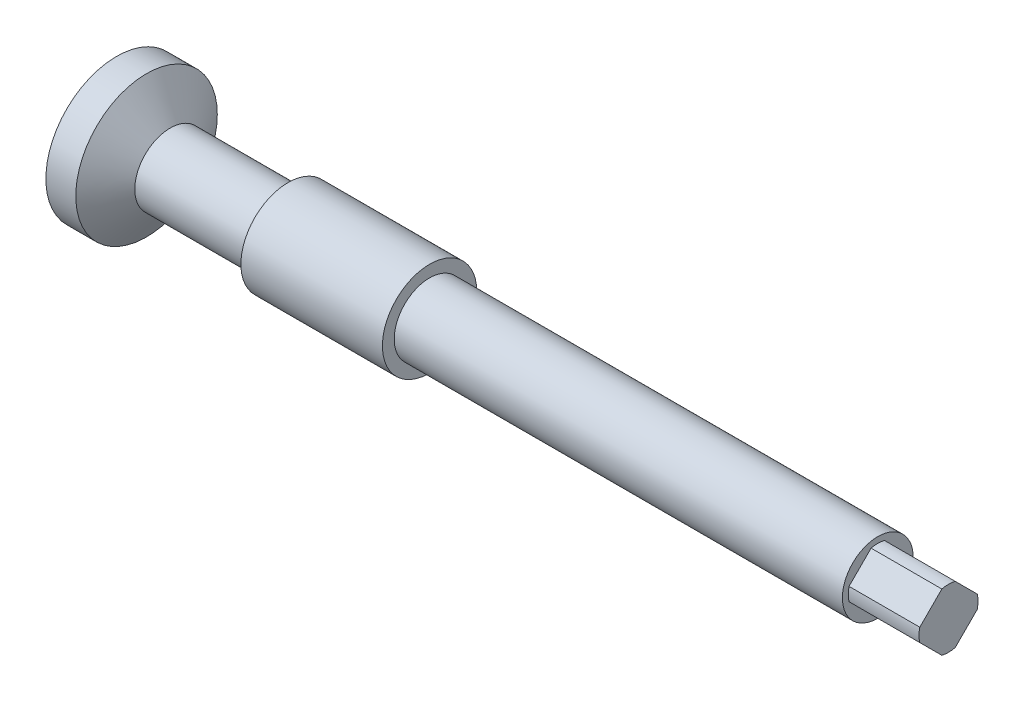
from build123d import *

# Parameters (mm, degrees)
SQUARE_DRIVE_SKETCH_OUTSIDE_W = 29.184
SQUARE_DRIVE_SKETCH_OUTSIDE_H = 29.184
SQUARE_DRIVE_5X5_CUT_DEPTH    = 6


with BuildPart() as part:
    # Spindle Profile Sketch → Spindle Body Revolve (revolve)
    with BuildSketch(Plane.XY, mode=Mode.PRIVATE) as spindle_body_revolve_sk:
        Polygon((0, 0), (0, 2.5), (-6, 2.5), (-6, 3), (-44, 3), (-44, 4), (-56, 4), (-56, 3), (-66, 3), (-68, 6), (-70.535898385, 6), (-74, 0), align=None)
    revolve(spindle_body_revolve_sk.sketch.rotate(Axis((0, 0, 0), (-1, 0, 0)), 90), axis=Axis((0, 0, 0), (-1, 0, 0)))

    # Square Drive Sketch outside → Square Drive 5x5 Cut (cut)
    with BuildSketch(Plane(origin=(0, 0, 0), x_dir=(0, 0, -1), z_dir=(1, 0, 0))):
        Rectangle(SQUARE_DRIVE_SKETCH_OUTSIDE_W, SQUARE_DRIVE_SKETCH_OUTSIDE_H)
        Polygon((-0.5, 2.5), (-2.5, 0.5), (-2.5, -0.5), (-0.5, -2.5), (0.5, -2.5), (2.5, -0.5), (2.5, 0.5), (0.5, 2.5), align=None, mode=Mode.SUBTRACT)
    extrude(amount=-SQUARE_DRIVE_5X5_CUT_DEPTH, mode=Mode.SUBTRACT)


solid = part.part
